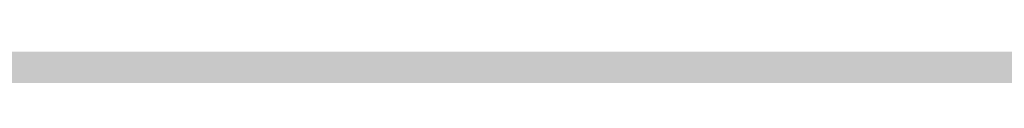
# Model space of a CAD drawing. Units: feet. Extents: x 3168 to 4724, y 827 to 1477.
# Tile 254 of 256: x 3384.42671 to 3384.48612, y 1099.01485 to 1099.01628. Entities that reach past the tile are written whole.
import ezdxf

# ---------------------------------------------------------------- set-up
doc = ezdxf.new("R2010")
doc.units = ezdxf.units.FT
doc.layers.add('A-ELEV', color=7, linetype='Continuous', lineweight=35)
doc.layers.add('A-ELEV-PATT', color=8, linetype='Continuous', lineweight=13)

msp = doc.modelspace()

# ---------------------------------------------------------------- hatches: boundary and pattern name
at = {"layer": 'A-ELEV-PATT'}
h = msp.add_hatch(color=256, dxfattribs=at)
h.dxf.hatch_style = 1
edge = h.paths.add_edge_path()
edge.add_ellipse((3552.905762, 979.220141), major_axis=(36.744924, 0), ratio=0.484848485, start_angle=0, end_angle=360)
edge = h.paths.add_edge_path()
edge.add_ellipse((3559.891637, 929.252282), major_axis=(36.744924, 0), ratio=0.484848485, start_angle=0, end_angle=360)
edge = h.paths.add_edge_path()
edge.add_line((3299.31681, 1198.606081), (3479.916714, 1198.606081))
edge.add_line((3479.916714, 1198.606081), (3479.916714, 1209.86857))
edge.add_spline(control_points=[(3479.916714, 1209.86857), (3464.301157, 1209.86857), (3448.685601, 1209.86857), (3410.949139, 1209.86857), (3388.828234, 1209.86857), (3355.646876, 1209.86857), (3344.586423, 1209.86857), (3327.995745, 1209.86857), (3322.465518, 1209.86857), (3314.170179, 1209.86857), (3311.405066, 1209.86857), (3307.257396, 1209.86857), (3305.874839, 1209.86857), (3303.801005, 1209.86857), (3303.109726, 1209.86857), (3302.072809, 1209.86857), (3301.72717, 1209.86857), (3301.208711, 1209.86857), (3301.035891, 1209.86857), (3300.776662, 1209.86857), (3300.690252, 1209.86857), (3300.560638, 1209.86857), (3300.517433, 1209.86857), (3300.452625, 1209.86857), (3300.431023, 1209.86857), (3300.398619, 1209.86857), (3300.387818, 1209.86857), (3300.366216, 1209.86857), (3300.345676, 1209.86857), (3300.345548, 1209.86857), (3300.345505, 1209.86857), (3300.343304, 1209.86857), (3300.341146, 1209.868571), (3300.337909, 1209.868571), (3300.33683, 1209.868572), (3300.333942, 1209.868573), (3300.332133, 1209.868574), (3300.325515, 1209.868577), (3300.320706, 1209.868581), (3300.310925, 1209.868592), (3300.305952, 1209.868598), (3300.290511, 1209.868623), (3300.280045, 1209.868646), (3300.232425, 1209.868777), (3300.195298, 1209.868954), (3299.951068, 1209.870608), (3299.744824, 1209.874326), (3299.436827, 1209.883257), (3299.334389, 1209.886792), (3299.181079, 1209.89292), (3299.130033, 1209.895099), (3298.652217, 1209.916801), (3298.22946, 1209.945718), (3297.601631, 1210.002367), (3297.393404, 1210.023464), (3297.082652, 1210.058309), (3296.979332, 1210.070458), (3296.292954, 1210.154861), (3295.718148, 1210.243356), (3294.868717, 1210.39885), (3294.5877, 1210.454478), (3294.169341, 1210.543349), (3294.030415, 1210.573878), (3291.707149, 1211.1012), (3289.65359, 1211.813435), (3285.776259, 1213.563988), (3283.95141, 1214.603478), (3280.512159, 1216.98008), (3278.897241, 1218.317592), (3276.379914, 1220.829489), (3275.416042, 1221.917738), (3274.039342, 1223.7077), (3273.581043, 1224.349535), (3273.143228, 1225.016316)], knot_values=[39.119033, 39.119033, 39.119033, 39.119033, 39.286353, 39.286353, 39.523379, 39.523379, 39.641892, 39.641892, 39.701148, 39.701148, 39.730777, 39.730777, 39.745591, 39.745591, 39.752998, 39.752998, 39.756701, 39.756701, 39.758553, 39.758553, 39.759479, 39.759479, 39.759942, 39.759942, 39.760173, 39.760173, 39.760289, 39.760289, 39.760405, 39.760405, 39.760463, 39.760463, 39.763389, 39.763389, 39.764851, 39.764851, 39.767304, 39.767304, 39.773825, 39.773825, 39.78057, 39.78057, 39.79477, 39.79477, 39.845194, 39.845194, 40.126715, 40.126715, 40.267476, 40.267476, 40.337856, 40.337856, 40.927023, 40.927023, 41.221606, 41.221606, 41.368898, 41.368898, 42.202622, 42.202622, 42.619485, 42.619485, 42.827916, 42.827916, 46.118323, 46.118323, 49.408731, 49.408731, 52.699139, 52.699139, 54.927489, 54.927489, 56.104228, 56.104228, 56.104228, 56.104228], weights=[1, 1, 1, 1, 1, 1, 1, 1, 1, 1, 1, 1, 1, 1, 1, 1, 1, 1, 1, 1, 1, 1, 1, 1, 1, 1, 1, 1, 1, 1, 1, 1, 1, 1, 1, 1, 1, 1, 1, 1, 1, 1, 1, 1, 1, 1, 1, 1, 1, 1, 1, 1, 1, 1, 1, 1, 1, 1, 1, 1, 1, 1, 1, 1, 1, 1, 1, 1, 1, 1, 1, 1, 1, 1], degree=3, periodic=0)
edge.add_line((3273.143228, 1225.016316), (3273.143228, 1099.016316))
edge.add_line((3273.143228, 1099.016316), (3299.31681, 1099.016316))
edge.add_line((3299.31681, 1099.016316), (3299.31681, 1198.606081))
edge = h.paths.add_edge_path()
edge.add_line((3304.758443, 1324.15806), (3479.916714, 1324.15806))
edge.add_line((3479.916714, 1324.15806), (3479.916714, 1335.714618))
edge.add_line((3479.916714, 1335.714618), (3269.161628, 1335.714618))
edge.add_spline(control_points=[(3269.161628, 1335.714618), (3264.024231, 1335.714618), (3258.364118, 1328.958189), (3259.264311, 1323.900274)], knot_values=[0, 0, 0, 0, 15.412191, 15.412191, 15.412191, 15.412191], degree=3, periodic=0)
edge.add_line((3259.264311, 1323.900274), (3265.516849, 1288.769135))
edge.add_line((3265.516849, 1288.769135), (3275.265103, 1261.545626))
edge.add_line((3275.265103, 1261.545626), (3304.758443, 1261.545626))
edge.add_line((3304.758443, 1261.545626), (3304.758443, 1324.15806))
h = msp.add_hatch(color=256, dxfattribs=at)
h.dxf.hatch_style = 1
h.paths.add_polyline_path([(3384.525247, 1099.016316), (3335.029168, 1099.016316), (3299.31681, 1099.016316), (3273.143228, 1099.016316), (3217.565364, 1099.016316), (3168.069285, 827.11626), (3335.029168, 827.11626)])

# ---------------------------------------------------------------- linework, layer by layer
at = {"layer": 'A-ELEV'}
msp.add_open_spline([(3808.5202, 1099.016316), (3808.5202, 1141.413235), (3808.5202, 1183.810154), (3808.5202, 1226.635324), (3808.5202, 1227.063576), (3808.5202, 1227.491828), (3811.491871, 1248.994673), (3814.463542, 1270.497518), (3817.46523, 1292.217564), (3817.495247, 1292.434764), (3817.525264, 1292.651964), (3817.572801, 1310.106748), (3817.620339, 1327.561532), (3817.667877, 1345.016316), (3817.667877, 1345.457962), (3817.667877, 1345.899608), (3817.667877, 1346.456047), (3817.667877, 1346.57084), (3817.667877, 1346.752887), (3817.667877, 1346.820142), (3817.667877, 1346.93487), (3817.667877, 1346.982345), (3817.667877, 1347.038587), (3817.667877, 1347.047356), (3817.667877, 1347.073661), (3817.667877, 1347.059303), (3817.667877, 1347.061545), (3817.667876, 1347.062667), (3817.667875, 1347.066031), (3817.667874, 1347.068274), (3817.66787, 1347.075001), (3817.667866, 1347.079486), (3817.667849, 1347.092937), (3817.667833, 1347.101902), (3817.667766, 1347.12879), (3817.667699, 1347.146705), (3817.667432, 1347.200421), (3817.667165, 1347.236192), (3817.6661, 1347.343385), (3817.665038, 1347.414686), (3817.660812, 1347.628095), (3817.656608, 1347.769708), (3817.63997, 1348.192487), (3817.623509, 1348.471586), (3817.559094, 1349.300067), (3817.496121, 1349.840588), (3817.255432, 1351.424156), (3817.026318, 1352.428785), (3816.306871, 1354.888914), (3815.743745, 1356.268727), (3814.463959, 1358.81921), (3813.746413, 1359.990968), (3812.195838, 1362.172343), (3811.362245, 1363.182124), (3809.588836, 1365.069009), (3808.648816, 1365.946105), (3806.654262, 1367.579616), (3805.599702, 1368.336154), (3803.352891, 1369.722327), (3802.160535, 1370.352386), (3799.600813, 1371.453586), (3798.232688, 1371.925481), (3795.280084, 1372.634624), (3793.693148, 1372.872068), (3791.869441, 1372.92648), (3791.740861, 1372.92922), (3791.353371, 1372.934101), (3791.092707, 1372.932901), (3790.304116, 1372.915068), (3789.769543, 1372.884195), (3789.20919, 1372.830236), (3789.190622, 1372.828424), (3789.134892, 1372.822912), (3789.097705, 1372.819137), (3789.048445, 1372.814008), (3789.0364, 1372.812743), (3789.000256, 1372.808918), (3788.976147, 1372.806325), (3788.949405, 1372.803404), (3788.946786, 1372.803118), (3788.942567, 1372.802655), (3788.940967, 1372.80248), (3788.938572, 1372.802217), (3788.937777, 1372.802129), (3788.935391, 1372.801867), (3788.867535, 1372.794402), (3788.756866, 1372.782228), (3788.701532, 1372.776141), (3788.53553, 1372.75788), (3788.424861, 1372.745707), (3788.092856, 1372.709185), (3787.871519, 1372.684837), (3787.207509, 1372.611793), (3786.764835, 1372.563097), (3785.436814, 1372.417009), (3784.551467, 1372.319617), (3781.895425, 1372.027442), (3780.12473, 1371.832658), (3774.812646, 1371.248307), (3771.271256, 1370.858739), (3760.647088, 1369.690037), (3753.56431, 1368.910902), (3732.315973, 1366.573498), (3718.150416, 1365.015228), (3694.006758, 1362.359326), (3684.028657, 1361.261694), (3674.050557, 1360.164062), (3664.600662, 1360.164062), (3655.150767, 1360.164062), (3626.801081, 1360.164062), (3607.901291, 1360.164062), (3551.20192, 1360.164062), (3513.40234, 1360.164062), (3467.725182, 1360.164062), (3459.847604, 1360.164062), (3436.214873, 1360.164062), (3420.459718, 1360.164062), (3373.194255, 1360.164062), (3341.683946, 1360.164062), (3302.848162, 1360.164062), (3295.522686, 1360.164062), (3286.038292, 1360.164062), (3283.879372, 1360.164062), (3277.402613, 1360.164062), (3273.084773, 1360.164062), (3267.732851, 1360.164062), (3266.698768, 1360.164062), (3263.59652, 1360.164062), (3261.528355, 1360.164062), (3259.236943, 1360.164062), (3259.013697, 1360.164062), (3258.343958, 1360.164062), (3257.897466, 1360.164062), (3257.430998, 1360.164062), (3257.411022, 1360.164062), (3257.370573, 1360.164062), (3257.37547, 1360.164062), (3257.374598, 1360.164062), (3257.373937, 1360.164062), (3257.371956, 1360.164062), (3257.370635, 1360.164061), (3257.366673, 1360.16406), (3257.364032, 1360.164059), (3257.356109, 1360.164053), (3257.350828, 1360.164047), (3257.334987, 1360.164023), (3257.32443, 1360.163998), (3257.292769, 1360.163899), (3257.271676, 1360.163799), (3257.208439, 1360.163398), (3257.166337, 1360.162995), (3257.040206, 1360.161388), (3256.956349, 1360.159783), (3256.705504, 1360.153393), (3256.53924, 1360.147036), (3256.04357, 1360.121916), (3255.717296, 1360.097102), (3254.752446, 1360.000481), (3254.127968, 1359.906513), (3252.180067, 1359.525332), (3250.941574, 1359.143991), (3248.670175, 1358.24329), (3247.635739, 1357.723834), (3245.732632, 1356.603471), (3244.863388, 1356.00206), (3243.253108, 1354.742865), (3242.511972, 1354.084731), (3240.751052, 1352.344781), (3239.800961, 1351.229574), (3238.087769, 1348.87244), (3237.324685, 1347.630355), (3235.98251, 1344.971632), (3235.402205, 1343.554907), (3234.591081, 1340.815458), (3234.310882, 1339.54355), (3233.97649, 1336.802561), (3233.922113, 1335.330877), (3234.148916, 1332.591269), (3234.349529, 1331.367201), (3234.719893, 1329.999367), (3234.752423, 1329.883362), (3234.853619, 1329.534797), (3234.925892, 1329.301685), (3235.024836, 1329.002552), (3235.046924, 1328.936928), (3235.077639, 1328.847239), (3235.085924, 1328.823198), (3235.110939, 1328.751064), (3235.127828, 1328.702962), (3235.147992, 1328.646242), (3235.151059, 1328.637632), (3235.156096, 1328.623526), (3235.158061, 1328.61803), (3235.160209, 1328.61203), (3235.165612, 1328.596943), (3235.180099, 1328.556486), (3235.190263, 1328.528101), (3235.220756, 1328.442946), (3235.241084, 1328.386176), (3235.302069, 1328.215865), (3235.342726, 1328.102325), (3235.464696, 1327.761704), (3235.54601, 1327.534623), (3235.78995, 1326.853381), (3235.952577, 1326.39922), (3236.440459, 1325.036736), (3236.765713, 1324.128414), (3237.741475, 1321.403446), (3238.391983, 1319.586801), (3240.343508, 1314.136866), (3241.644525, 1310.503576), (3245.547574, 1299.603706), (3248.149607, 1292.337126), (3255.955706, 1270.537385), (3261.159772, 1256.004225), (3267.387618, 1238.612001), (3268.411397, 1235.752937), (3269.510378, 1232.683864), (3269.585579, 1232.473854), (3269.706612, 1232.135851), (3269.752444, 1232.007857), (3269.827329, 1231.79873), (3269.856382, 1231.717595), (3269.906325, 1231.578122), (3269.927215, 1231.519782), (3269.972468, 1231.393406), (3269.996831, 1231.325368), (3270.026503, 1231.242506), (3270.031811, 1231.227681), (3270.040282, 1231.204024), (3270.039224, 1231.206979), (3270.039359, 1231.206601), (3270.039427, 1231.206412), (3270.03963, 1231.205846), (3270.039765, 1231.205468), (3270.040171, 1231.204335), (3270.040442, 1231.203579), (3270.041254, 1231.201313), (3270.041796, 1231.199802), (3270.04342, 1231.195269), (3270.044504, 1231.192248), (3270.047756, 1231.183185), (3270.049926, 1231.177145), (3270.056442, 1231.159028), (3270.060793, 1231.146957), (3270.073867, 1231.110761), (3270.082613, 1231.086656), (3270.108936, 1231.014413), (3270.1266, 1230.96635), (3270.179934, 1230.822457), (3270.215947, 1230.726923), (3270.325323, 1230.441508), (3270.400026, 1230.252811), (3270.629249, 1229.691444), (3270.788883, 1229.323501), (3271.286488, 1228.238319), (3271.6431, 1227.539755), (3272.775859, 1225.515277), (3273.614169, 1224.260502), (3275.416042, 1221.917738), (3276.379914, 1220.829489), (3278.897241, 1218.317592), (3280.512159, 1216.98008), (3283.95141, 1214.603478), (3285.776259, 1213.563988), (3289.65359, 1211.813435), (3291.707149, 1211.1012), (3294.030415, 1210.573878), (3294.169341, 1210.543349), (3294.5877, 1210.454478), (3294.868717, 1210.39885), (3295.718148, 1210.243356), (3296.292954, 1210.154861), (3296.979332, 1210.070458), (3297.082652, 1210.058309), (3297.393404, 1210.023464), (3297.601631, 1210.002367), (3298.22946, 1209.945718), (3298.652217, 1209.916801), (3299.130033, 1209.895099), (3299.181079, 1209.89292), (3299.334389, 1209.886792), (3299.436827, 1209.883257), (3299.744824, 1209.874326), (3299.951068, 1209.870608), (3300.195298, 1209.868954), (3300.232425, 1209.868777), (3300.280045, 1209.868646), (3300.290511, 1209.868623), (3300.305952, 1209.868598), (3300.310925, 1209.868592), (3300.320706, 1209.868581), (3300.325515, 1209.868577), (3300.332133, 1209.868574), (3300.333942, 1209.868573), (3300.33683, 1209.868572), (3300.337909, 1209.868571), (3300.341146, 1209.868571), (3300.343304, 1209.86857), (3300.345505, 1209.86857), (3300.345548, 1209.86857), (3300.345676, 1209.86857), (3300.366216, 1209.86857), (3300.387818, 1209.86857), (3300.398619, 1209.86857), (3300.431023, 1209.86857), (3300.452625, 1209.86857), (3300.517433, 1209.86857), (3300.560638, 1209.86857), (3300.690252, 1209.86857), (3300.776662, 1209.86857), (3301.035891, 1209.86857), (3301.208711, 1209.86857), (3301.72717, 1209.86857), (3302.072809, 1209.86857), (3303.109726, 1209.86857), (3303.801005, 1209.86857), (3305.874839, 1209.86857), (3307.257396, 1209.86857), (3311.405066, 1209.86857), (3314.170179, 1209.86857), (3322.465518, 1209.86857), (3327.995745, 1209.86857), (3344.586423, 1209.86857), (3355.646876, 1209.86857), (3388.828234, 1209.86857), (3410.949139, 1209.86857), (3477.311855, 1209.86857), (3521.553665, 1209.86857), (3566.836184, 1209.86857), (3567.876892, 1209.86857), (3570.999017, 1209.86857), (3573.080433, 1209.86857), (3575.781396, 1209.86857), (3576.400943, 1209.86857), (3577.295821, 1209.86857), (3577.571152, 1209.86857), (3578.397146, 1209.86857), (3578.947808, 1209.86857), (3579.756491, 1209.86857), (3580.014511, 1209.86857), (3580.342737, 1209.86857), (3580.326865, 1209.86857), (3580.32717, 1209.86857), (3580.327323, 1209.86857), (3580.327781, 1209.86857), (3580.328086, 1209.86857), (3580.329002, 1209.86857), (3580.329613, 1209.86857), (3580.331445, 1209.86857), (3580.332667, 1209.86857), (3580.336332, 1209.868569), (3580.338775, 1209.868567), (3580.346107, 1209.868563), (3580.350995, 1209.868558), (3580.365663, 1209.86854), (3580.375445, 1209.868522), (3580.404801, 1209.868449), (3580.424386, 1209.868376), (3580.483183, 1209.868085), (3580.522437, 1209.867793), (3580.640361, 1209.866624), (3580.719195, 1209.865454), (3580.956315, 1209.860766), (3581.115222, 1209.85607), (3581.594164, 1209.83723), (3581.916419, 1209.818331), (3582.889947, 1209.742428), (3583.547986, 1209.666169), (3585.531827, 1209.360617), (3586.867216, 1209.053886), (3589.471545, 1208.252472), (3590.740241, 1207.757852), (3591.995451, 1207.158802), (3592.057809, 1207.12874), (3592.244242, 1207.037954), (3592.367676, 1206.976632), (3592.73528, 1206.790359), (3592.976752, 1206.663101), (3593.244539, 1206.516441), (3593.274731, 1206.499825), (3593.365115, 1206.449839), (3593.425113, 1206.416333), (3593.604314, 1206.315285), (3593.722725, 1206.247211), (3593.857212, 1206.168398), (3593.874362, 1206.158319), (3593.925741, 1206.128041), (3593.959899, 1206.107798), (3594.062086, 1206.046899), (3594.129827, 1206.006074), (3594.208436, 1205.958171), (3594.219683, 1205.951304), (3594.253391, 1205.930686), (3594.275819, 1205.916917), (3594.342972, 1205.875536), (3594.387563, 1205.847853), (3594.433616, 1205.81905), (3594.435256, 1205.818024), (3594.440175, 1205.814946), (3594.443453, 1205.812894), (3594.447123, 1205.810594), (3594.447516, 1205.810348), (3594.448695, 1205.80961), (3594.449481, 1205.809117), (3594.450366, 1205.808562), (3594.450466, 1205.8085), (3594.4506, 1205.808415), (3594.467399, 1205.797887), (3594.493269, 1205.781674), (3594.506204, 1205.773568), (3594.545008, 1205.749248), (3594.570878, 1205.733035), (3594.648487, 1205.684396), (3594.700226, 1205.651969), (3594.855444, 1205.554691), (3594.958922, 1205.489839), (3595.269357, 1205.295282), (3595.476314, 1205.165577), (3596.097185, 1204.776463), (3596.511099, 1204.517054), (3597.752841, 1203.738826), (3598.580669, 1203.220007), (3601.064152, 1201.663551), (3602.719807, 1200.625914), (3607.686774, 1197.513002), (3610.998085, 1195.437727), (3620.932018, 1189.211903), (3627.55464, 1185.061354), (3647.422507, 1172.609707), (3660.667751, 1164.308608), (3700.403484, 1139.405313), (3726.893973, 1122.803116), (3757.205715, 1103.806052), (3761.02697, 1101.411184), (3764.848224, 1099.016316), (3745.328271, 1099.016316), (3725.808319, 1099.016316), (3706.288366, 1099.016316), (3706.288366, 1108.453237), (3706.288366, 1117.890158), (3706.288366, 1127.327079), (3710.750754, 1127.327079), (3715.213143, 1127.327079), (3719.675531, 1127.327079)], degree=3, knots=[0, 0, 0, 0, 0.982037, 0.982037, 0.991957, 0.991957, 0.991957, 1.966522, 1.966522, 1.976367, 1.976367, 1.976367, 2.976367, 2.976367, 2.976367, 3.00169, 3.00169, 3.008272, 3.008272, 3.012129, 3.012129, 3.014851, 3.014851, 3.015353, 3.015353, 3.016359, 3.016359, 3.017365, 3.017365, 3.019376, 3.019376, 3.023398, 3.023398, 3.031442, 3.031442, 3.047531, 3.047531, 3.079708, 3.079708, 3.144063, 3.144063, 3.272772, 3.272772, 3.53019, 3.53019, 4.045026, 4.045026, 5.074698, 5.074698, 6.700878, 6.700878, 8.327058, 8.327058, 9.953238, 9.953238, 11.579418, 11.579418, 13.205598, 13.205598, 14.831778, 14.831778, 16.457958, 16.457958, 18.084138, 18.084138, 18.206872, 18.206872, 18.45234, 18.45234, 18.943275, 18.943275, 18.960093, 18.960093, 18.993729, 18.993729, 19.00461, 19.00461, 19.026374, 19.026374, 19.028737, 19.028737, 19.03018, 19.03018, 19.030897, 19.030897, 19.032332, 19.032332, 19.033766, 19.033766, 19.036636, 19.036636, 19.042374, 19.042374, 19.053851, 19.053851, 19.076805, 19.076805, 19.122714, 19.122714, 19.21453, 19.21453, 19.398163, 19.398163, 19.765429, 19.765429, 20.024128, 20.024128, 20.024128, 20.092031, 20.092031, 20.227836, 20.227836, 20.499446, 20.499446, 20.556051, 20.556051, 20.66926, 20.66926, 20.895678, 20.895678, 20.948316, 20.948316, 20.963829, 20.963829, 20.994855, 20.994855, 21.002285, 21.002285, 21.017146, 21.017146, 21.01875, 21.01875, 21.021959, 21.021959, 21.022102, 21.022102, 21.022249, 21.022249, 21.022708, 21.022708, 21.023627, 21.023627, 21.025464, 21.025464, 21.029138, 21.029138, 21.036486, 21.036486, 21.051183, 21.051183, 21.080575, 21.080575, 21.139361, 21.139361, 21.256932, 21.256932, 21.492073, 21.492073, 21.962356, 21.962356, 23.01002, 23.01002, 24.057684, 24.057684, 25.105348, 25.105348, 26.153011, 26.153011, 27.776787, 27.776787, 29.400562, 29.400562, 31.024337, 31.024337, 32.278801, 32.278801, 33.533265, 33.533265, 34.467568, 34.467568, 34.553971, 34.553971, 34.726776, 34.726776, 34.775309, 34.775309, 34.793079, 34.793079, 34.82862, 34.82862, 34.834979, 34.834979, 34.839039, 34.839039, 34.839411, 34.839411, 34.840285, 34.840285, 34.842034, 34.842034, 34.845531, 34.845531, 34.852525, 34.852525, 34.866512, 34.866512, 34.894488, 34.894488, 34.950439, 34.950439, 35.062342, 35.062342, 35.286147, 35.286147, 35.733758, 35.733758, 35.821815, 35.821815, 35.828283, 35.828283, 35.832225, 35.832225, 35.834724, 35.834724, 35.836521, 35.836521, 35.838617, 35.838617, 35.839073, 35.839073, 35.839345, 35.839345, 35.839617, 35.839617, 35.840161, 35.840161, 35.841249, 35.841249, 35.843425, 35.843425, 35.847778, 35.847778, 35.856482, 35.856482, 35.873891, 35.873891, 35.908709, 35.908709, 35.978345, 35.978345, 36.117617, 36.117617, 36.396161, 36.396161, 36.953248, 36.953248, 38.067423, 38.067423, 40.295772, 40.295772, 42.524122, 42.524122, 45.81453, 45.81453, 49.104937, 49.104937, 52.395345, 52.395345, 52.603776, 52.603776, 53.020639, 53.020639, 53.854363, 53.854363, 54.001655, 54.001655, 54.296238, 54.296238, 54.885405, 54.885405, 54.955785, 54.955785, 55.096546, 55.096546, 55.378067, 55.378067, 55.42849, 55.42849, 55.442691, 55.442691, 55.449436, 55.449436, 55.455957, 55.455957, 55.458409, 55.458409, 55.459872, 55.459872, 55.462798, 55.462798, 55.462856, 55.462856, 55.462972, 55.462972, 55.463088, 55.463088, 55.463319, 55.463319, 55.463782, 55.463782, 55.464708, 55.464708, 55.46656, 55.46656, 55.470263, 55.470263, 55.47767, 55.47767, 55.492484, 55.492484, 55.522112, 55.522112, 55.581369, 55.581369, 55.699882, 55.699882, 55.936907, 55.936907, 56.410959, 56.410959, 56.42211, 56.42211, 56.444413, 56.444413, 56.451051, 56.451051, 56.454001, 56.454001, 56.459901, 56.459901, 56.462666, 56.462666, 56.463418, 56.463418, 56.464171, 56.464171, 56.465675, 56.465675, 56.468684, 56.468684, 56.474702, 56.474702, 56.486738, 56.486738, 56.51081, 56.51081, 56.558955, 56.558955, 56.655243, 56.655243, 56.847821, 56.847821, 57.232975, 57.232975, 58.003284, 58.003284, 59.543901, 59.543901, 62.625137, 62.625137, 68.787607, 68.787607, 74.950078, 74.950078, 75.27336, 75.27336, 75.919923, 75.919923, 77.213051, 77.213051, 77.377769, 77.377769, 77.707206, 77.707206, 78.366079, 78.366079, 78.462532, 78.462532, 78.655436, 78.655436, 79.041245, 79.041245, 79.105735, 79.105735, 79.234714, 79.234714, 79.492672, 79.492672, 79.502197, 79.502197, 79.521249, 79.521249, 79.523534, 79.523534, 79.528103, 79.528103, 79.528682, 79.528682, 79.528885, 79.528885, 79.529089, 79.529089, 79.529495, 79.529495, 79.530308, 79.530308, 79.531935, 79.531935, 79.535187, 79.535187, 79.541693, 79.541693, 79.554704, 79.554704, 79.580725, 79.580725, 79.632769, 79.632769, 79.736856, 79.736856, 79.94503, 79.94503, 80.361377, 80.361377, 80.421435, 80.421435, 80.421435, 81.421435, 81.421435, 81.421435, 82.421435, 82.421435, 82.421435, 83.421435, 83.421435, 83.421435, 83.421435], dxfattribs=at)

doc.saveas('drawing.dxf')
